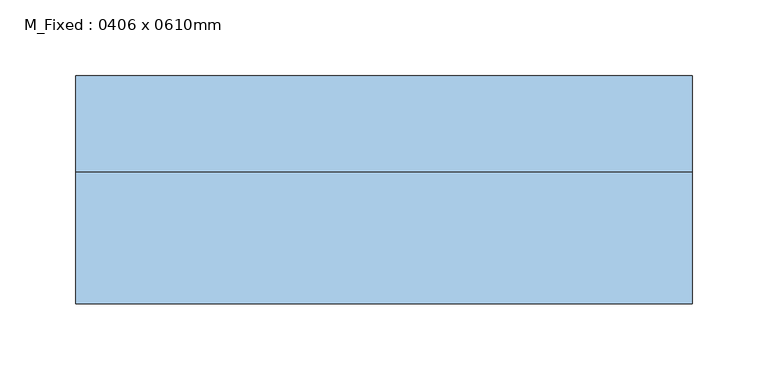
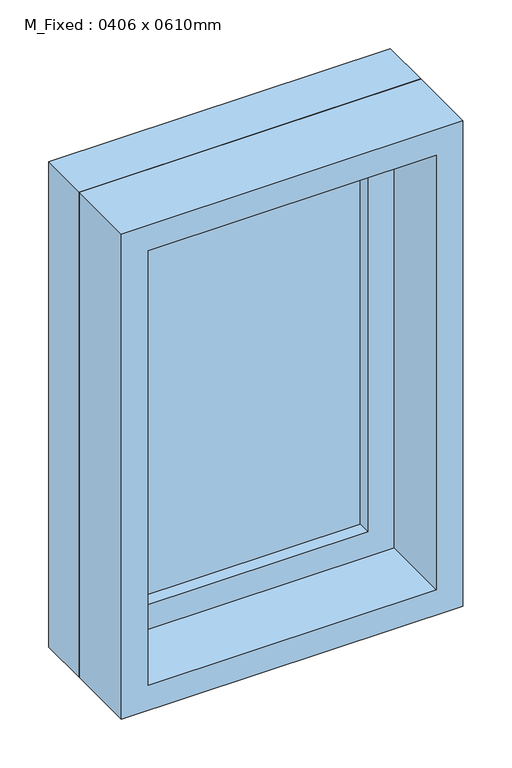
"""IFC4 building model written with IfcOpenShell, lengths in millimetres: window geometry, M_Fixed : 0406 x 0610mm."""

from ifc_helpers import new_model, si_unit, frame, origin, place, context, project, spatial, polyline, outline, extrude, source, transform, mapped, element, save


def m_fixed_0406_x_0610mm_893b2dd9(model_context):
    return source(origin(), model_context, "Body", "SweptSolid", [
        extrude(outline(polyline([(-140.0, 53.0), (140.0, 53.0), (140.0, 41.0), (-140.0, 41.0), (-140.0, 53.0)])), frame((0.0, 0.0, 978.0), z_axis=(0.0, 0.0, 1.0), x_axis=(1.0, 0.0, 0.0)), (0.0, 0.0, 1.0), 484.0),
        extrude(outline(polyline([(1506.0, -184.0), (934.0, -184.0), (934.0, 184.0), (1506.0, 184.0), (1506.0, -184.0)]), holes=[polyline([(1462.0, -140.0), (1462.0, 140.0), (978.0, 140.0), (978.0, -140.0), (1462.0, -140.0)])]), frame((0.0, 25.0, 0.0), z_axis=(0.0, 1.0, 0.0), x_axis=(0.0, 0.0, 1.0)), (0.0, 0.0, 1.0), 44.0),
        extrude(outline(polyline([(1525.0, -203.0), (915.0, -203.0), (915.0, 203.0), (1525.0, 203.0), (1525.0, -203.0)]), holes=[polyline([(1506.0, -184.0), (1506.0, 184.0), (934.0, 184.0), (934.0, -184.0), (1506.0, -184.0)])]), frame((0.0, 25.0, 0.0), z_axis=(0.0, 1.0, 0.0), x_axis=(0.0, 0.0, 1.0)), (0.0, 0.0, 1.0), 63.0),
        extrude(outline(polyline([(1525.0, -203.0), (915.0, -203.0), (915.0, 203.0), (1525.0, 203.0), (1525.0, -203.0)]), holes=[polyline([(1493.0, -171.0), (1493.0, 171.0), (947.0, 171.0), (947.0, -171.0), (1493.0, -171.0)])]), frame((0.0, -62.0, 0.0), z_axis=(0.0, 1.0, 0.0), x_axis=(0.0, 0.0, 1.0)), (0.0, 0.0, 1.0), 87.0),
    ])


if __name__ == "__main__":
    model = new_model("IFC4")
    model_context = context("Model", 3, world=origin())
    ifc_project = project(units=[si_unit("LENGTHUNIT", "METRE", prefix="MILLI")], contexts=[model_context])
    site = spatial("IfcSite", under=ifc_project)
    building = spatial("IfcBuilding", under=site)
    placement = place(None, origin())
    m_fixed_0406_x_0610mm_shape = m_fixed_0406_x_0610mm_893b2dd9(model_context)
    element("IfcWindow", 1, ObjectType="M_Fixed : 0406 x 0610mm", at=placement, inside=building, context=model_context, shape_type="MappedRepresentation", body=[
        mapped(m_fixed_0406_x_0610mm_shape, transform((0.0, 0.0, 0.0), x_axis=(1.0, 0.0, 0.0), y_axis=(0.0, 1.0, 0.0), z_axis=(0.0, 0.0, 1.0))),
    ])
    save(model, "model.ifc")

# Revit data of these elements
# Type "M_Fixed : 0406 x 0610mm"
#   Type Mark = "10"
#   Height = 610 mm
#   Default Sill Height = 915 mm
#   Width = 406 mm
#   Window Inset = 19 mm
#   Frame Exterior Material = Sash
#   Frame Interior Material = Sash
#   Glass Pane Material = Glass
#   Sash = Sash
#   Wall Closure = (empty or 0)
# Element 1 (IfcWindow, "M_Fixed : 0406 x 0610mm")
#   Materials on its faces: "Sash", "Glass"
# Materials
#   "Sash": class "Wood", colour RGB 136 99 55, transparency 0
#   "Glass": class "Glass", colour RGB 218 227 224, transparency 0.85, Description = "Soda Lime Glass", Cost = 0
